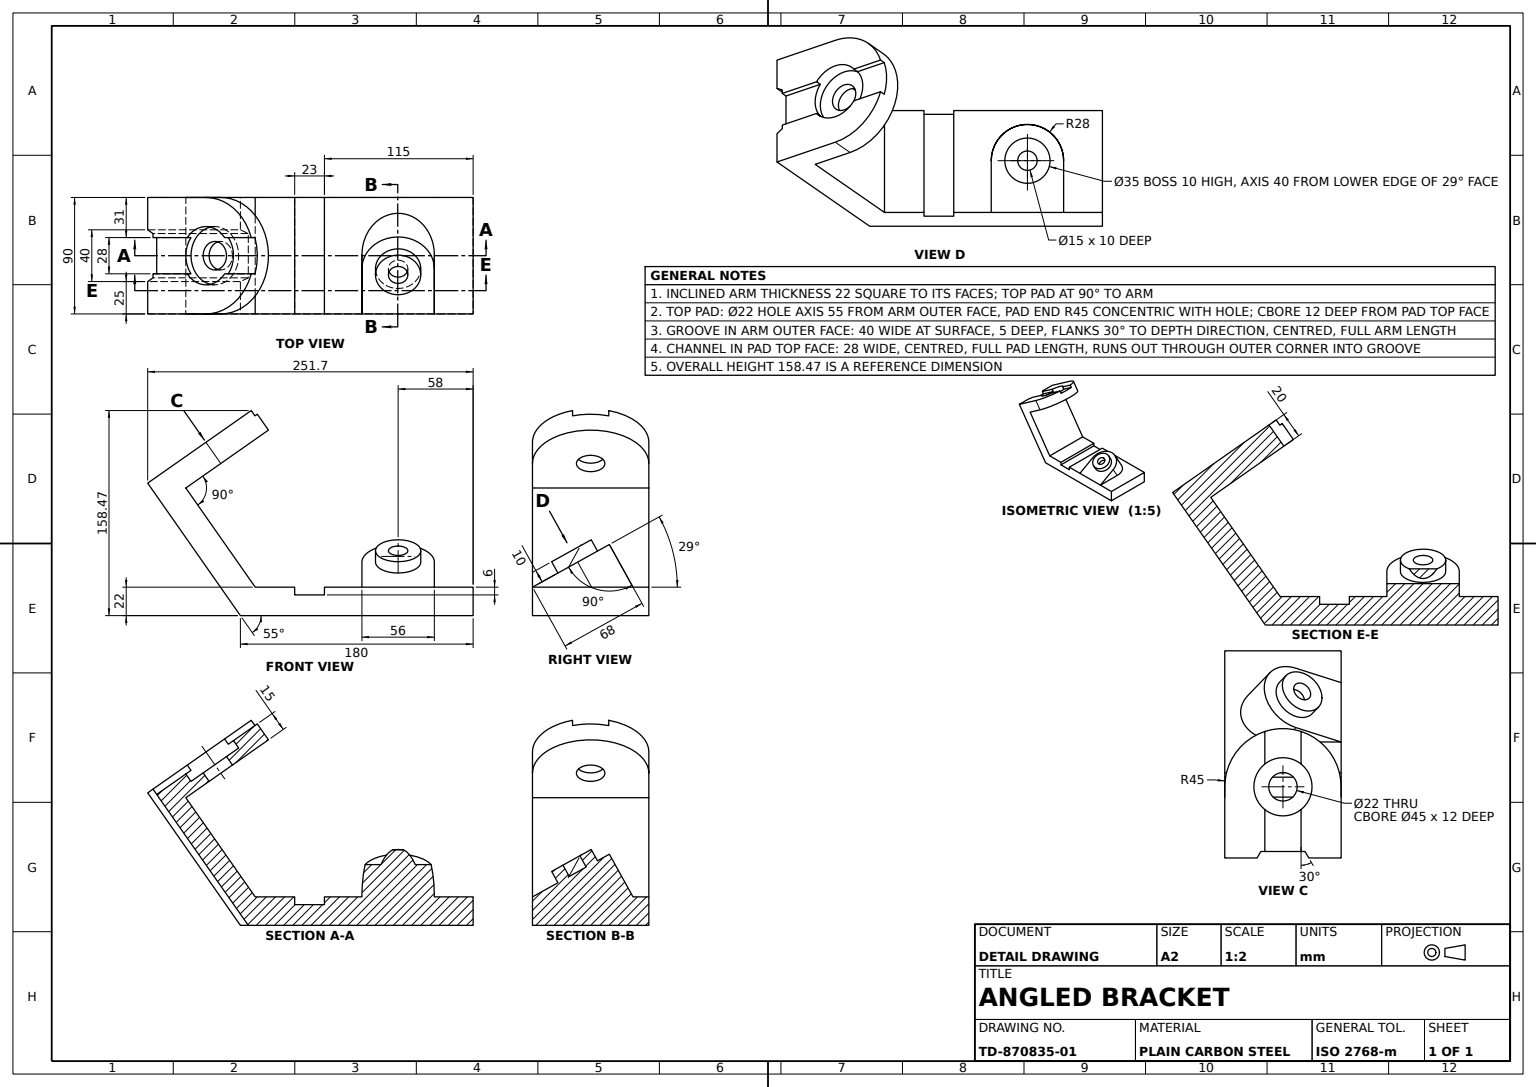
from build123d import *

# Parameters (mm, degrees)
BASE_PLATE_SKETCH_W        = 180
BASE_PLATE_SKETCH_H        = 90
BASE_PLATE_180X90X22_DEPTH = 22
INCLINED_BOSS_BLOCK_REACH  = 118.629
PIVOT_BOSS_SKETCH_R        = 17.5
PIVOT_BOSS_SKETCH_R_2      = 7.5
PIVOT_BOSS_DEPTH           = 10
CROSS_SLOT_SKETCH_W        = 23
CROSS_SLOT_SKETCH_H        = 90
CROSS_SLOT_23X6_DEPTH      = 6
UPRIGHT_ARM_SKETCH_W       = 90
UPRIGHT_ARM_SKETCH_H       = 125
INCLINED_UPRIGHT_ARM_DEPTH = 22
TOP_PAD_DEPTH              = 20
C_BORE_HOLE_22_D           = 22
C_BORE_HOLE_22_DEPTH       = 22.19797288
C_BORE_HOLE_22_CBORE_D     = 45
C_BORE_HOLE_22_CBORE_DEPTH = 12
TOP_PAD_NOTCHES_DEPTH      = 245.0397404
CROSS_RECESS_SKETCH_W      = 32.386085046
CROSS_RECESS_SKETCH_H      = 28
CROSS_RECESS_SKETCH_W_2    = 30
CROSS_RECESS_5_DEEP_DEPTH  = 5


with BuildPart() as part:
    # Base Plate Sketch → Base Plate 180x90x22 (new body)
    with BuildSketch(Plane(origin=(0, 0, 0), x_dir=(1, 0, 0), z_dir=(0, 1, 0))):
        Rectangle(BASE_PLATE_SKETCH_W, BASE_PLATE_SKETCH_H)
    extrude(amount=BASE_PLATE_180X90X22_DEPTH)

    # Inclined Boss Block Sketch → Inclined Boss Block (add, up to next)
    with BuildSketch(Plane(origin=(0, 35.91019407, 19.905345612), x_dir=(-1, 0, 0), z_dir=(0, -0.874619707139395, -0.48480962024633867)), mode=Mode.PRIVATE) as inclined_boss_block_sk1:
        with BuildLine():
            Line((-4, 11.307924824), (-4, -28.692075176))
            Line((-4, -28.692075176), (-60, -28.692075176))
            Line((-60, -28.692075176), (-60, 11.307924824))
            ThreePointArc((-60, 11.307924824), (-32, 39.307924824), (-4, 11.307924824))
        make_face()
    inclined_boss_block_tool1 = extrude(inclined_boss_block_sk1.sketch, amount=INCLINED_BOSS_BLOCK_REACH, mode=Mode.PRIVATE) - part.part
    add(inclined_boss_block_tool1.solids().sort_by_distance((32, 37.179674, 17.615143))[0])

    # Pivot Boss Sketch → Pivot Boss (add)
    with BuildSketch(Plane(origin=(0, 35.91019407, 19.905345612), x_dir=(1, 0, 0), z_dir=(0, 0.8746197071393949, 0.4848096202463387))):
        with Locations(Location((32, 11.307924824, 0), (0, 0, 90))):
            Circle(PIVOT_BOSS_SKETCH_R)
        with Locations(Location((32, 11.307924824, 0), (0, 0, 270))):
            Circle(PIVOT_BOSS_SKETCH_R_2, mode=Mode.SUBTRACT)
    extrude(amount=PIVOT_BOSS_DEPTH)

    # Cross Slot Sketch → Cross Slot 23x6 (cut)
    with BuildSketch(Plane(origin=(0, 22, 0), x_dir=(1, 0, 0), z_dir=(0, 1, 0))):
        with Locations((-36.5, 0)):
            Rectangle(CROSS_SLOT_SKETCH_W, CROSS_SLOT_SKETCH_H)
    extrude(amount=-CROSS_SLOT_23X6_DEPTH, mode=Mode.SUBTRACT)

    # Upright Arm Sketch → Inclined Upright Arm (add)
    with BuildSketch(Plane(origin=(-60.39090645, -42.286167935, 0), x_dir=(0, 0, -1), z_dir=(0.8191520442889931, 0.5735764363510442, 0))):
        with Locations((0, 114.121879272)):
            Rectangle(UPRIGHT_ARM_SKETCH_W, UPRIGHT_ARM_SKETCH_H)
    extrude(amount=INCLINED_UPRIGHT_ARM_DEPTH)

    # Top Pad Sketch → Top Pad (add)
    with BuildSketch(Plane(origin=(-101.306148094, 144.680173471, 0), x_dir=(0.8191520442889931, 0.5735764363510442, 0), z_dir=(-0.5735764363510442, 0.8191520442889931, 0))):
        with BuildLine():
            Line((-18.723683986, 45), (-73.723683986, 45))
            Line((-73.723683986, 45), (-73.723683986, -45))
            Line((-73.723683986, -45), (-18.723683986, -45))
            ThreePointArc((-18.723683986, -45), (26.276316014, 0), (-18.723683986, 45))
        make_face()
    extrude(amount=-TOP_PAD_DEPTH)

    # C-Bore Hole Ø22
    with Locations(Plane(origin=(-101.306148094, 144.680173471, 0), x_dir=(0.8191520442889931, 0.5735764363510442, 0), z_dir=(-0.5735764363510442, 0.8191520442889931, 0))):
        with Locations((-18.723683986, 0)):
            CounterBoreHole(C_BORE_HOLE_22_D / 2, C_BORE_HOLE_22_CBORE_D / 2, C_BORE_HOLE_22_CBORE_DEPTH, depth=C_BORE_HOLE_22_DEPTH)

    # Top Pad Notch Sketch → Top Pad Notches (cut, through all)
    with BuildSketch(Plane(origin=(-101.306148094, 144.680173471, 0), x_dir=(0.8191520442889931, 0.5735764363510442, 0), z_dir=(-0.5735764363510442, 0.8191520442889931, 0))):
        Polygon((-73.723683986, 20), (-68.723683986, 17.113248654), (-68.723683986, -17.113248654), (-73.723683986, -20), align=None)
    extrude(amount=-TOP_PAD_NOTCHES_DEPTH, mode=Mode.SUBTRACT)

    # Cross Recess Sketch → Cross Recess 5 Deep (cut)
    with BuildSketch(Plane(origin=(-101.306148094, 144.680173471, 0), x_dir=(0.8191520442889931, 0.5735764363510442, 0), z_dir=(-0.5735764363510442, 0.8191520442889931, 0))):
        with Locations((-52.530641463, 0)):
            Rectangle(CROSS_RECESS_SKETCH_W, CROSS_RECESS_SKETCH_H)
        with Locations((13.890230968, 0)):
            Rectangle(CROSS_RECESS_SKETCH_W_2, CROSS_RECESS_SKETCH_H)
    extrude(amount=-CROSS_RECESS_5_DEEP_DEPTH, mode=Mode.SUBTRACT)


solid = part.part
